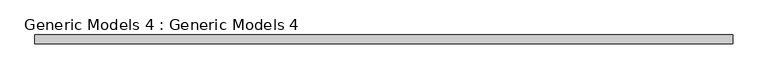
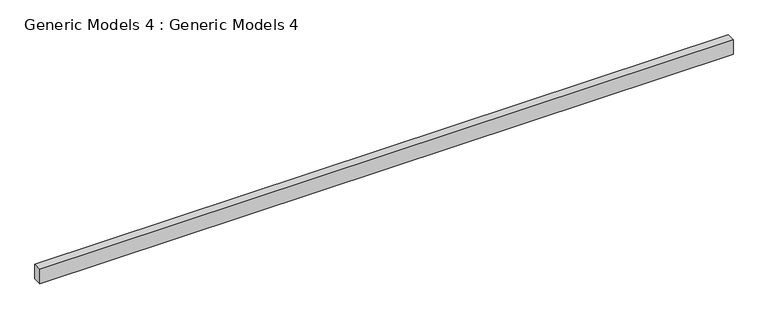
"""IFC4 building model written with IfcOpenShell, lengths in millimetres: proxy geometry, Generic Models 4 : Generic Models 4."""

from ifc_helpers import new_model, si_unit, frame, origin, place, context, project, spatial, polyline, outline, extrude, source, transform, mapped, element, save


def generic_models_4_generic_models_4_7fc0937d(model_context):
    return source(origin(), model_context, "Body", "SweptSolid", [
        extrude(outline(polyline([(12604.4370151, -3682.5004242), (12604.4370151, -3955.4201358), (-8934.7629849, -3955.4201358), (-8934.7629849, -3682.5004242), (12604.4370151, -3682.5004242)])), frame((0.0, 0.0, 6210.1291394), z_axis=(0.0, 0.0, 1.0), x_axis=(1.0, 0.0, 0.0)), (0.0, 0.0, 1.0), 468.4331878),
    ])


if __name__ == "__main__":
    model = new_model("IFC4")
    model_context = context("Model", 3, world=origin())
    ifc_project = project(units=[si_unit("LENGTHUNIT", "METRE", prefix="MILLI")], contexts=[model_context])
    site = spatial("IfcSite", under=ifc_project)
    building = spatial("IfcBuilding", under=site)
    placement = place(None, origin())
    generic_models_4_generic_models_4_shape = generic_models_4_generic_models_4_7fc0937d(model_context)
    element("IfcBuildingElementProxy", 1, Name="Generic Models 4 : Generic Models 4", ObjectType="Generic Models 4 : Generic Models 4", at=placement, inside=building, context=model_context, shape_type="MappedRepresentation", body=[
        mapped(generic_models_4_generic_models_4_shape, transform((0.0, 0.0, 0.0), x_axis=(1.0, 0.0, 0.0), y_axis=(0.0, 1.0, 0.0), z_axis=(0.0, 0.0, 1.0))),
    ])
    save(model, "model.ifc")
